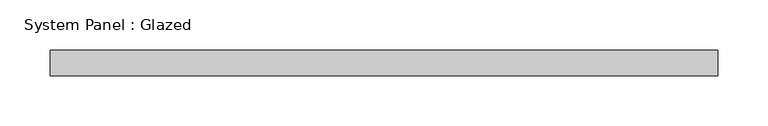
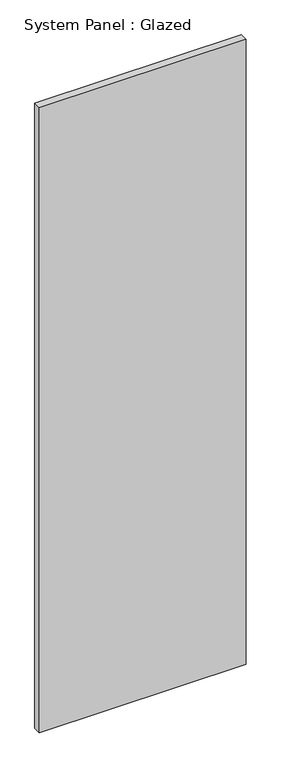
"""IFC4 building model written with IfcOpenShell, lengths in millimetres: plate geometry, System Panel : Glazed."""

from ifc_helpers import new_model, si_unit, origin, origin_with_axes, place, context, project, spatial, polyline, outline, extrude, source, transform, mapped, element, save


def system_panel_glazed_8c1b86c6(model_context):
    return source(origin(), model_context, "Body", "SweptSolid", [
        extrude(outline(polyline([(333.375, 19.05), (-333.375, 19.05), (-333.375, 44.45), (333.375, 44.45), (333.375, 19.05)])), origin_with_axes(), (0.0, 0.0, 1.0), 2132.5340877),
    ])


if __name__ == "__main__":
    model = new_model("IFC4")
    model_context = context("Model", 3, world=origin())
    ifc_project = project(units=[si_unit("LENGTHUNIT", "METRE", prefix="MILLI")], contexts=[model_context])
    site = spatial("IfcSite", under=ifc_project)
    building = spatial("IfcBuilding", under=site)
    placement = place(None, origin())
    system_panel_glazed_shape = system_panel_glazed_8c1b86c6(model_context)
    element("IfcPlate", 1, ObjectType="System Panel : Glazed", at=placement, inside=building, context=model_context, shape_type="MappedRepresentation", body=[
        mapped(system_panel_glazed_shape, transform((0.0, 0.0, 0.0), x_axis=(1.0, 0.0, 0.0), y_axis=(0.0, 1.0, 0.0), z_axis=(0.0, 0.0, 1.0))),
    ])
    save(model, "model.ifc")

# Revit data of these elements
# Type "System Panel : Glazed"
#   Construction Type Id = "GSP4R"
#   Analytic Construction = "1/8 in Pilkington single glazing"
#   Visual Light Transmittance = 0.9
#   Solar Heat Gain Coefficient = 0.86
#   Heat Transfer Coefficient (U) = 1.18115 BTU/(h·ft²·°F)
# Element 1 (IfcPlate, "System Panel : Glazed")
#   Materials on its faces: "Glass"
# Materials
#   "Glass": class "Glass", colour RGB 0 128 192, transparency 0.75, Description = "Soda Lime Glass", Cost = 0
